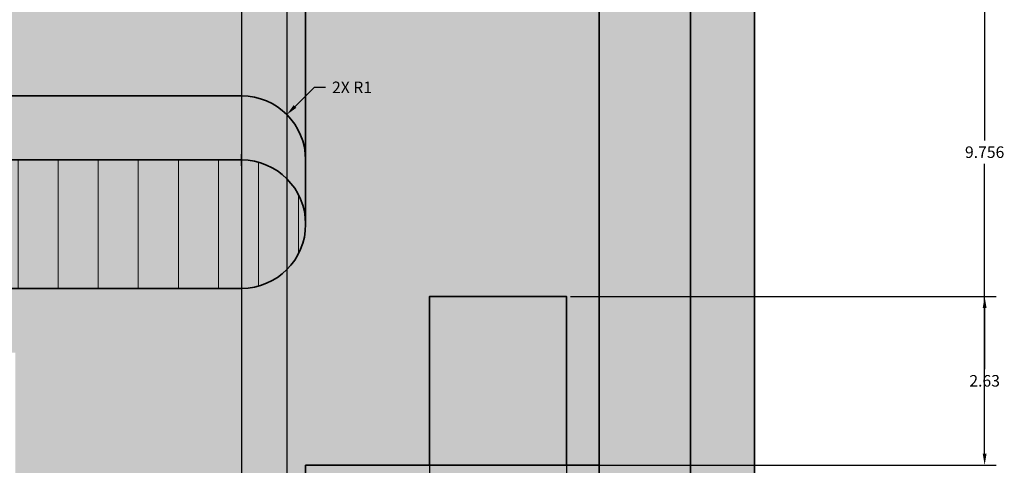
# Model space of a CAD drawing. Units: inches. Extents: x 18 to 59.8, y 2.7 to 81.2.
# Tile 6 of 9: x 44.4 to 59.8, y 38.7 to 45.6. Entities that reach past the tile are written whole.
import ezdxf

# ---------------------------------------------------------------- set-up
doc = ezdxf.new("R2010")
doc.units = ezdxf.units.IN
doc.header["$MEASUREMENT"] = 0
for name, color, linetype, lineweight in [('A-ANNO-DIMS', 2, 'Continuous', 18), ('A-ELEV', 7, 'Continuous', 35), ('A-ELEV-PATT', 8, 'Continuous', 13)]:
    doc.layers.add(name, color=color, linetype=linetype, lineweight=lineweight)
doc.styles.get("Standard").update_dxf_attribs({"font": 'arial.ttf'})
doc.dimstyles.get("Standard").update_dxf_attribs({"dimtxt": 0.18, "dimasz": 0.18, "dimexe": 0.18, "dimexo": 0.0625, "dimgap": 0.09, "dimtad": 0, "dimtih": 1, "dimtoh": 1, "dimdec": 1, "dimzin": 0, "dimdsep": 46, "dimlunit": 3, "dimtxsty": 'Standard', "dimcen": 0.09, "dimadec": 0, "dimazin": 0, "dimtfac": 1, "dimtdec": 1, "dimtofl": 0, "dimtmove": 0, "dimatfit": 3, "dimfxl": 1, "dimtolj": 1, "dimtzin": 0, "dimarcsym": 0})

# ---------------------------------------------------------------- blocks, each defined once
blk = doc.blocks.new('*D17')
at = {"layer": 'A-ANNO-DIMS', "color": 0, "lineweight": -2, "transparency": 16777216}
for p, q in [((53.50256100000002, 48.44074800000003), (59.62997100000005, 48.44074800000003)), ((59.44997100000005, 48.26074800000003), (59.44997100000005, 43.74455863778991)), ((59.44997100000005, 38.86456300000001), (59.44997100000005, 43.38075236221011)), ((53.50256100000002, 38.68456300000001), (59.62997100000006, 38.68456300000001))]:
    blk.add_line(p, q, dxfattribs=at)
at = {"layer": 'A-ANNO-DIMS', "color": 0, "transparency": 16777216}
for points in [[(59.41997100000005, 48.26074800000003), (59.47997100000005, 48.26074800000003), (59.44997100000005, 48.44074800000003)], [(59.41997100000005, 38.86456300000001), (59.47997100000005, 38.86456300000001), (59.44997100000005, 38.68456300000001)]]:
    blk.add_solid(points, dxfattribs=at)
at = {"layer": 'Defpoints', "color": 0, "transparency": 16777216}
for p in [(53.44006100000003, 48.44074800000003), (59.44997100000005, 48.44074800000003), (53.44006100000003, 38.68456300000001)]:
    blk.add_point(p, dxfattribs=at)
at = {"layer": 'A-ANNO-DIMS', "color": 0, "transparency": 16777216, "insert": (59.44997100000005, 43.56265549999998), "char_height": 0.18, "attachment_point": 5}
blk.add_mtext('\\A1;9.756', dxfattribs=at)
blk = doc.blocks.new('*D25')
at = {"layer": 'A-ANNO-DIMS', "color": 0, "lineweight": -2, "transparency": 16777216}
for p, q in [((50.792976, 41.253458), (50.792976, 2.670748000000003)), ((52.926966, 41.253458), (52.926966, 2.670748000000003)), ((50.972976, 2.850747999999999), (51.46510060436562, 2.850747999999999)), ((52.746966, 2.850747999999999), (52.25484139563437, 2.850747999999999))]:
    blk.add_line(p, q, dxfattribs=at)
at = {"layer": 'A-ANNO-DIMS', "color": 0, "transparency": 16777216}
for points in [[(50.972976, 2.880747999999999), (50.972976, 2.820748), (50.792976, 2.850747999999999)], [(52.746966, 2.880747999999999), (52.746966, 2.820748), (52.926966, 2.850747999999999)]]:
    blk.add_solid(points, dxfattribs=at)
at = {"layer": 'Defpoints', "color": 0, "transparency": 16777216}
for p in [(50.792976, 41.315958), (52.926966, 41.315958), (52.926966, 2.850747999999999)]:
    blk.add_point(p, dxfattribs=at)
at = {"layer": 'A-ANNO-DIMS', "color": 0, "transparency": 16777216, "insert": (51.859971, 2.850747999999999), "char_height": 0.18, "attachment_point": 5}
blk.add_mtext('\\A1;2.134', dxfattribs=at)
blk = doc.blocks.new('*D26')
at = {"layer": 'A-ANNO-DIMS', "color": 0, "lineweight": -2, "transparency": 16777216}
for p, q in [((52.98946600000003, 41.31595800000002), (59.62997100000006, 41.31595800000002)), ((59.44997100000005, 41.13595800000001), (59.44997100000005, 40.18222502933153)), ((59.44997100000005, 38.86456300000001), (59.44997100000005, 39.8182959706685)), ((52.98946600000003, 38.68456300000001), (59.62997100000006, 38.68456300000001))]:
    blk.add_line(p, q, dxfattribs=at)
at = {"layer": 'A-ANNO-DIMS', "color": 0, "transparency": 16777216}
for points in [[(59.41997100000005, 41.13595800000001), (59.47997100000005, 41.13595800000001), (59.44997100000005, 41.31595800000002)], [(59.41997100000005, 38.86456300000001), (59.47997100000005, 38.86456300000001), (59.44997100000005, 38.68456300000001)]]:
    blk.add_solid(points, dxfattribs=at)
at = {"layer": 'Defpoints', "color": 0, "transparency": 16777216}
for p in [(52.92696600000002, 41.31595800000002), (59.44997100000005, 41.31595800000002), (52.92696600000002, 38.68456300000001)]:
    blk.add_point(p, dxfattribs=at)
at = {"layer": 'A-ANNO-DIMS', "color": 0, "transparency": 16777216, "insert": (59.44997100000005, 40.00026049999998), "char_height": 0.18, "attachment_point": 5}
blk.add_mtext('\\A1;2.63', dxfattribs=at)
blk = doc.blocks.new('*D51')
at = {"layer": 'A-ANNO-DIMS', "color": 0, "lineweight": -2, "transparency": 16777216}
for p, q in [((34.011642, 44.50324799999999), (34.011642, 81.210748)), ((48.859971, 43.503248), (48.859971, 81.210748)), ((34.191642, 81.03074799999999), (40.98046543587994, 81.03074799999999)), ((48.679971, 81.03074799999999), (41.89114756412005, 81.03074799999999))]:
    blk.add_line(p, q, dxfattribs=at)
at = {"layer": 'A-ANNO-DIMS', "color": 0, "transparency": 16777216}
for points in [[(34.191642, 81.060748), (34.191642, 81.00074799999999), (34.011642, 81.03074799999999)], [(48.679971, 81.060748), (48.679971, 81.00074799999999), (48.859971, 81.03074799999999)]]:
    blk.add_solid(points, dxfattribs=at)
at = {"layer": 'Defpoints', "color": 0, "transparency": 16777216}
for p in [(48.859971, 81.03074799999999), (34.011642, 44.440748), (48.859971, 43.440748)]:
    blk.add_point(p, dxfattribs=at)
at = {"layer": 'A-ANNO-DIMS', "color": 0, "transparency": 16777216, "insert": (41.43580649999999, 81.03074799999999), "char_height": 0.18, "attachment_point": 5}
blk.add_mtext('\\A1;14.848', dxfattribs=at)
blk = doc.blocks.new('*D61')
at = {"layer": 'A-ANNO-DIMS', "color": 0, "lineweight": -2, "transparency": 16777216}
for p, q in [((32.233824, 49.378248), (32.233824, 2.670748000000003)), ((47.859971, 49.378248), (47.859971, 2.670748000000003)), ((32.413824, 2.850747999999999), (39.59180200204638, 2.850747999999999)), ((47.679971, 2.850747999999999), (40.50199299795361, 2.850747999999999))]:
    blk.add_line(p, q, dxfattribs=at)
at = {"layer": 'A-ANNO-DIMS', "color": 0, "transparency": 16777216}
for points in [[(32.413824, 2.880747999999999), (32.413824, 2.820748), (32.233824, 2.850747999999999)], [(47.679971, 2.880747999999999), (47.679971, 2.820748), (47.859971, 2.850747999999999)]]:
    blk.add_solid(points, dxfattribs=at)
at = {"layer": 'Defpoints', "color": 0, "transparency": 16777216}
for p in [(32.233824, 49.440748), (47.859971, 49.440748), (47.859971, 2.850747999999999)]:
    blk.add_point(p, dxfattribs=at)
at = {"layer": 'A-ANNO-DIMS', "color": 0, "transparency": 16777216, "insert": (40.04689749999999, 2.850747999999999), "char_height": 0.18, "attachment_point": 5}
blk.add_mtext('\\A1;15.626', dxfattribs=at)
blk = doc.blocks.new('*D66')
at = {"layer": 'A-ANNO-DIMS', "color": 0, "lineweight": -2, "transparency": 16777216}
for p, q in [((28.803543, 51.378248), (28.803543, 2.670748000000003)), ((48.567078, 51.179103), (48.567078, 2.670748000000003)), ((28.983543, 2.850747999999999), (38.23052195975444, 2.850747999999999)), ((48.387078, 2.850747999999999), (39.14009904024556, 2.850747999999999))]:
    blk.add_line(p, q, dxfattribs=at)
at = {"layer": 'A-ANNO-DIMS', "color": 0, "transparency": 16777216}
for points in [[(28.983543, 2.880747999999999), (28.983543, 2.820748), (28.803543, 2.850747999999999)], [(48.387078, 2.880747999999999), (48.387078, 2.820748), (48.567078, 2.850747999999999)]]:
    blk.add_solid(points, dxfattribs=at)
at = {"layer": 'Defpoints', "color": 0, "transparency": 16777216}
for p in [(28.803543, 51.440748), (48.567078, 51.24160299999999), (48.567078, 2.850747999999999)]:
    blk.add_point(p, dxfattribs=at)
at = {"layer": 'A-ANNO-DIMS', "color": 0, "transparency": 16777216, "insert": (38.6853105, 2.850747999999999), "char_height": 0.18, "attachment_point": 5}
blk.add_mtext('\\A1;19.764', dxfattribs=at)
blk = doc.blocks.new('*D71')
at = {"layer": 'A-ANNO-DIMS', "color": 0, "lineweight": -2, "transparency": 16777216}
for p, q in [((48.99116316341159, 44.57229696346312), (48.6942251490235, 44.27526528903896)), ((49.17116316341159, 44.57229696346312), (48.99116316341159, 44.57229696346312)), ((47.859971, 43.35074800000001), (47.859971, 43.53074800000001)), ((47.769971, 43.44074800000001), (47.94997099999999, 43.44074800000001))]:
    blk.add_line(p, q, dxfattribs=at)
at = {"layer": 'A-ANNO-DIMS', "color": 0, "transparency": 16777216}
blk.add_solid([(48.67300860085034, 44.29647514720953), (48.71544169719665, 44.25405543086838), (48.56696600000001, 44.14796600000001)], dxfattribs=at)
at = {"layer": 'Defpoints', "color": 0, "transparency": 16777216}
for p in [(48.56696600000001, 44.14796600000001), (47.859971, 43.44074800000001)]:
    blk.add_point(p, dxfattribs=at)
at = {"layer": 'A-ANNO-DIMS', "color": 0, "transparency": 16777216, "insert": (49.58383710611282, 44.57229696346312), "char_height": 0.18, "attachment_point": 5}
blk.add_mtext('\\A1;2X R1', dxfattribs=at)

msp = doc.modelspace()

# ---------------------------------------------------------------- hatches: boundary and pattern name
at = {"layer": 'A-ELEV-PATT'}
h = msp.add_hatch(color=256, dxfattribs=at)
h.set_gradient(color1=(255, 255, 255), color2=(199, 200, 202))
h.paths.add_polyline_path([(38.85997087182833, 75.45212783007513, 0.4125526599533602), (36.85997087192615, 77.44074750583997), (21.85997087182832, 77.44074750583995), (21.85997087182832, 22.44074750583995), (22.85997087182833, 22.44074750583995), (48.85997087182833, 22.44074750583996), (48.85997087182833, 30.92342676155402, 0.4074472928332927), (48.33023903111634, 31.44074750583995), (30.40609029701442, 31.44074750583996, -0.7603989452129261), (34.01164157247843, 44.44074750583996), (47.85997087182832, 44.44074750583995, -0.4142135623730951), (48.85997087182833, 43.44074750583994), (48.85997087182833, 48.44074750583995, 0.4142135623730955), (47.85997087182832, 49.44074750583995), (32.23382408177119, 49.44074750583993, -0.2243141867862321), (27.84111392101349, 52.84266085519661, -0.8480128940945467), (38.85997087182833, 61.44074750583993)])
h.paths.add_polyline_path([(55.85997087182832, 77.44074750583995), (54.85997087182832, 77.44074750583997), (54.85997087182832, 22.24074750583996), (55.85997087182832, 22.24074750583995)])
h.paths.add_polyline_path([(54.85997087182832, 51.54074750583995), (53.44006084017791, 51.54074750583996), (53.44006084017792, 29.64074750583996), (54.85997087182832, 29.64074750583996)])
h.paths.add_polyline_path([(54.85997087182832, 61.44074750583993), (53.44006084017791, 57.44074750583993), (53.44006084017791, 51.64074750583996), (54.85997087182832, 51.64074750583996)])
h.paths.add_polyline_path([(54.85997087182832, 29.44074750583995), (54.47100875861361, 29.44074750583995), (54.47100875861361, 22.24074750583996), (54.85997087182832, 22.24074750583996)])
h.paths.add_polyline_path([(55.57447446325177, 22.24074750583995), (54.85997087182832, 22.24074750583996), (54.57447446325178, 22.24074750583996), (53.93466996146642, 21.792542566958), (54.58769880335594, 21.54947740208223)])
h.paths.add_polyline_path([(54.59913950424823, 21.54521903603421), (53.94430429933965, 21.78895655088426), (53.94430429933965, 18.44074750583995), (54.59913950424823, 18.44074750583995)])
h.paths.add_polyline_path([(53.94430429933965, 21.78895655088427), (53.93466996146642, 21.792542566958), (53.58162006229036, 21.54521903603422), (53.58162006229036, 18.44074750583995), (53.94430429933965, 18.44074750583994)])
h.paths.add_polyline_path([(53.36475139777029, 20.69276091189374), (52.89555240690669, 21.06460517556268), (52.89555240690669, 18.44074750583995), (53.3647513977703, 18.44074750583994)])
h.paths.add_polyline_path([(52.89555240690669, 21.06460517556268), (50.57752474318004, 19.44074750583995), (50.57752474318004, 18.44074750583995), (52.89555240690669, 18.44074750583995)])
h.paths.add_polyline_path([(53.58162006229036, 21.54521903603423), (52.89555240690668, 21.06460517556268), (53.3647513977703, 20.69276091189373), (53.58162006229036, 20.84468482967704)])
h.paths.add_polyline_path([(26.81093959479239, 19.44074750583995), (24.96715419074249, 20.84074750583995), (24.96715419074249, 18.44074750583995), (26.81093959479239, 18.44074750583995)])
h.paths.add_polyline_path([(24.96715419074249, 20.84074750583995), (24.41645576890079, 20.84268308307895), (24.41645576890079, 18.44074750583994), (24.96715419074249, 18.44074750583994)])
h.paths.add_polyline_path([(24.41645576890079, 20.84268308307895), (24.41645576890079, 21.25889692219009), (24.05877847081848, 21.5304839605815), (24.03006070560372, 21.51834150822755), (24.03006070560372, 18.44074750583995), (24.41645576890079, 18.44074750583995)])
h.paths.add_polyline_path([(24.03006070560372, 21.51834150822755), (23.41645576890078, 21.2588969221901), (23.41645576890078, 18.44074750583996), (24.03006070560372, 18.44074750583995)])
h.paths.add_polyline_path([(24.03006070560372, 21.51834150822755), (24.05877847081849, 21.53048396058151), (23.12336878669258, 22.24074750583995), (22.12336878669259, 22.24074750583996), (23.41645576890079, 21.2588969221901)])
h.paths.add_polyline_path([(24.41645576890079, 21.2588969221901), (24.41645576890079, 20.84268308307896), (24.96715419074249, 20.84074750583994)])
h.paths.add_polyline_path([(47.85997087182832, 18.44074750583995), (29.85997087182832, 18.44074750583995), (29.85997087182832, 6.440747505839951), (30.85997087182832, 6.440747505839937), (30.85997087182832, 17.44074750583995), (38.85997087182833, 17.44074750583995), (46.85997087182832, 17.44074750583995), (46.85997087182832, 6.440747505839937), (47.85997087182832, 6.440747505839958)])
h.paths.add_polyline_path([(54.57559250001032, 15.2149800477124), (54.57559250001032, 6.440747505839944), (55.85997087182832, 6.440747505839951), (55.85997087182832, 18.44074750583995), (47.85997087182832, 18.44074750583995), (47.85997087182832, 6.440747505839944), (49.14824210254597, 6.440747505839944), (49.14824210254597, 15.2149800477124, -1)])
h = msp.add_hatch(color=256, dxfattribs=at)
h.paths.add_polyline_path([(27.84111392101356, 52.84266085519647, -0.7443789445921651), (36.85997087182832, 61.44074750583993), (38.85997087182833, 61.44074750583993, 0.8480128940945556)])
h.paths.add_polyline_path([(47.85997087182832, 44.44074750583995), (34.01164157247843, 44.44074750583996, 0.7603989452129407), (30.40609029701462, 31.44074750583983, -0.7376245609052545), (34.01164157247731, 43.44074750583994), (47.85997087182831, 43.44074750583994, -0.4142135623730951), (48.85997087182832, 42.44074750583995), (48.85997087182833, 43.44074750583994, 0.4142135623730951)])
h.paths.add_polyline_path([(54.57559250001032, 15.2149800477124), (54.57559250001032, 6.440747505839951), (55.85997087182832, 6.440747505839951), (55.85997087182832, 18.44074750583995), (47.85997087182832, 18.44074750583995), (47.85997087182832, 6.440747505839944), (49.14824210254597, 6.440747505839944), (49.14824210254597, 15.2149800477124, -1)])
h.paths.add_polyline_path([(47.85997087182832, 18.44074750583995), (29.85997087182832, 18.44074750583995), (29.85997087182832, 6.440747505839958), (30.85997087182832, 6.440747505839951), (30.85997087182832, 17.44074750583995), (38.85997087182833, 17.44074750583995), (46.85997087182832, 17.44074750583995), (46.85997087182832, 6.440747505839944), (47.85997087182832, 6.440747505839951)])
h.paths.add_polyline_path([(55.85997087182832, 77.44074750583995), (54.85997087182832, 77.44074750583997), (54.85997087182833, 22.24074750583995), (55.85997087182832, 22.24074750583995)])
h = msp.add_hatch(color=256, dxfattribs=at)
h.dxf.hatch_style = 1
h.paths.add_polyline_path([(54.85997087182832, 69.44074750583995), (38.85997087182833, 69.44074750583995), (38.85997087182833, 61.44074750583995), (54.85997087182832, 61.44074750583994)])
h.paths.add_polyline_path([(54.85997087182833, 61.44074750583994), (38.85997087182833, 61.44074750583995), (36.85997087182832, 61.44074750583993, 0.4434140223301819), (27.69861713021859, 58.44074750583995), (48.85997087182833, 58.44074750583995), (48.85997087182833, 57.44074750583994), (53.44006084017792, 57.44074750583995)])
h.paths.add_polyline_path([(37.49943513222304, 59.93991004599954), (37.49943513222304, 59.81982440572959, -2.410649922227508), (37.11866134610267, 59.81982440572959), (37.11866134610267, 59.93991004599954)], flags=16)
h.paths.add_polyline_path([(42.61253184194623, 59.80122867549901), (42.61253184194623, 59.92131431576897), (42.9933056280666, 59.92131431576897), (42.9933056280666, 59.80122867549901, -2.410649922227521)], flags=16)
h.paths.add_polyline_path([(49.59651616109447, 59.97095150496527), (49.59651616109447, 60.09103714523522), (49.97728994721485, 60.09103714523522), (49.97728994721485, 59.97095150496527, -2.410649922227521)], flags=16)
h.paths.add_polyline_path([(44.46707765301489, 57.04074750583994), (32.6670776530149, 57.04074750583994), (32.6670776530149, 56.04074750583993), (44.46707765301489, 56.04074750583993)])
h.paths.add_polyline_path([(47.85997087182831, 43.44074750583994), (46.85997087182832, 43.44074750583994), (34.0116415724774, 43.44074750583994, 0.2012982920418866), (29.34810857035394, 41.44074750583995), (47.85997087182831, 41.44074750583995, 1)])
h.paths.add_polyline_path([(36.55415719635351, 42.51454569609198), (36.55415719635351, 42.63463133636193), (36.93493098247388, 42.63463133636193), (36.93493098247388, 42.51454569609198, -2.410649922227513)], flags=16)
h.paths.add_polyline_path([(42.93899993637245, 42.54016758592221), (42.93899993637245, 42.66025322619216), (43.31977372249282, 42.66025322619216), (43.31977372249282, 42.54016758592221, -2.410649922227521)], flags=16)
h.paths.add_polyline_path([(54.47100875861361, 29.44074750583995), (48.85997087182833, 29.44074750583995), (48.85997087182833, 22.24074750583995), (54.47100875861361, 22.24074750583995)])
h.paths.add_polyline_path([(54.57447446325178, 22.24074750583996), (23.12336878669258, 22.24074750583996), (26.81093959479238, 19.44074750583996), (50.57752474318006, 19.44074750583996)])
h.paths.add_polyline_path([(54.57559250001032, 15.2149800477124, 1), (49.14824210254597, 15.2149800477124), (49.14824210254597, 6.440747505839958), (54.57559250001032, 6.440747505839965)])
h.paths.add_polyline_path([(49.83226884926398, 12.6020427608384), (49.83226884926398, 9.122455521673542), (49.66565363924473, 9.122455521673537), (49.66565363924473, 12.6020427608384)], flags=16)
h = msp.add_hatch(dxfattribs=at)
h.set_pattern_fill('ANSI31', color=256, scale=5, angle=45, style=0)
h.set_pattern_definition([(90, (0, 0), (-0.6250000000000001, 0), [])])
h.paths.add_polyline_path([(54.85997087182832, 69.44074750583995), (38.85997087182833, 69.44074750583995), (38.85997087182833, 61.44074750583995), (54.85997087182832, 61.44074750583994)])
h.paths.add_polyline_path([(54.85997087182833, 61.44074750583994), (38.85997087182833, 61.44074750583995), (36.85997087182832, 61.44074750583993, 0.4434140223301819), (27.69861713021859, 58.44074750583995), (48.85997087182833, 58.44074750583995), (48.85997087182833, 57.44074750583994), (53.44006084017792, 57.44074750583995)])
h.paths.add_polyline_path([(37.16613704638868, 59.85769359025997), (37.11866134610267, 59.85769359025997), (37.11866134610267, 59.93991004599954), (37.49943513222304, 59.93991004599954), (37.49943513222304, 59.85769359025997), (37.45195943193702, 59.85769359025997, -3.476462016968403)], flags=16)
h.paths.add_polyline_path([(42.66000754223224, 59.8390978600294), (42.61253184194623, 59.8390978600294), (42.61253184194623, 59.92131431576897), (42.9933056280666, 59.92131431576897), (42.9933056280666, 59.8390978600294), (42.94582992778058, 59.8390978600294, -3.47646201696846)], flags=16)
h.paths.add_polyline_path([(49.64399186138049, 60.00882068949565), (49.59651616109447, 60.00882068949565), (49.59651616109447, 60.09103714523522), (49.97728994721485, 60.09103714523522), (49.97728994721485, 60.00882068949565), (49.92981424692883, 60.00882068949565, -3.476462016968434)], flags=16)
h.paths.add_polyline_path([(44.46707765301489, 57.04074750583994), (32.6670776530149, 57.04074750583994), (32.6670776530149, 56.04074750583993), (44.46707765301489, 56.04074750583993)])
h.paths.add_polyline_path([(47.85997087182831, 43.44074750583994), (46.85997087182832, 43.44074750583994), (34.0116415724774, 43.44074750583994, 0.2012982920418866), (29.34810857035394, 41.44074750583995), (47.85997087182831, 41.44074750583995, 1)])
h.paths.add_polyline_path([(36.60163289663952, 42.55241488062237), (36.55415719635351, 42.55241488062236), (36.55415719635351, 42.63463133636193), (36.93493098247388, 42.63463133636193), (36.93493098247388, 42.55241488062236), (36.88745528218787, 42.55241488062236, -3.476462016968307)], flags=16)
h.paths.add_polyline_path([(42.98647563665846, 42.5780367704526), (42.93899993637245, 42.5780367704526), (42.93899993637245, 42.66025322619216), (43.31977372249282, 42.66025322619216), (43.31977372249282, 42.57803677045259), (43.2722980222068, 42.57803677045259, -3.476462016968351)], flags=16)
h.paths.add_polyline_path([(54.47100875861361, 29.44074750583995), (48.85997087182833, 29.44074750583995), (48.85997087182833, 22.24074750583995), (54.47100875861361, 22.24074750583994)])
h.paths.add_polyline_path([(54.57447446325179, 22.24074750583995), (23.12336878669258, 22.24074750583995), (26.81093959479238, 19.44074750583996), (50.57752474318005, 19.44074750583996)])
h.paths.add_polyline_path([(54.57559250001032, 15.2149800477124, 1), (49.14824210254597, 15.2149800477124), (49.14824210254597, 6.440747505839958), (54.57559250001032, 6.440747505839944)])
h.paths.add_polyline_path([(49.83226884926398, 9.122455521673542), (49.66565363924473, 9.122455521673537), (49.66565363924473, 12.60204276083839), (49.83226884926398, 12.6020427608384)], flags=16)
at = {"layer": 'A-ELEV-PATT', "transparency": 33554620}
h = msp.add_hatch(color=256, dxfattribs=at)
h.set_gradient(color1=(147, 149, 152))
edge = h.paths.add_edge_path()
edge.add_line((32.5670776530149, 55.94074750583994), (32.5670776530149, 57.14074750583994))
edge.add_line((32.5670776530149, 57.14074750583994), (44.5670776530149, 57.14074750583994))
edge.add_line((44.5670776530149, 57.14074750583994), (44.5670776530149, 55.94074750583994))
edge.add_line((44.5670776530149, 55.94074750583994), (44.56707765301487, 51.54074750583998))
edge.add_line((44.56707765301487, 51.54074750583998), (47.92075940082271, 51.54074750583998))
edge.add_spline(control_points=[(47.92075940082271, 51.54074750583998), (48.15238228194087, 51.51452682454292), (48.35972996747788, 51.37806491819363), (48.56707765301488, 51.24160301184435)], knot_values=[0, 0, 0, 0, 0.7121900809507601, 0.7121900809507601, 0.7121900809507601, 0.7121900809507601], degree=3, periodic=0)
edge.add_line((48.56707765301488, 51.24160301184435), (48.56707765301488, 49.14785428702649))
edge.add_arc((47.85997087182832, 48.44074750583995), 1, 5.739170477267294, 44.999999999999375, ccw=False)
edge.add_line((48.85495830893494, 48.54074750583996), (48.85997087182833, 48.54074750583996))
edge.add_line((48.85997087182833, 48.54074750583996), (48.85997087182833, 49.44074750583995))
edge.add_line((48.85997087182833, 49.44074750583995), (48.85997087182833, 58.44074750583995))
edge.add_line((48.85997087182833, 58.44074750583995), (27.6986171302186, 58.44074750583995))
edge.add_arc((33.63815495998532, 55.79107886226907), 6.503756879831279, 155.9580213816849, 220.80747886606)
edge.add_line((28.71539791616241, 51.54074750583994), (32.5670776530149, 51.54074750583994))
edge.add_line((32.5670776530149, 51.54074750583994), (32.5670776530149, 55.94074750583994))
edge = h.paths.add_edge_path()
edge.add_line((32.33023903111487, 40.44074750583996), (35.33023903111486, 40.44074750583996))
edge.add_line((35.33023903111486, 40.44074750583996), (38.33023903111485, 40.44074750583996))
edge.add_line((38.33023903111485, 40.44074750583996), (41.33023903111483, 40.44074750583996))
edge.add_line((41.33023903111483, 40.44074750583996), (44.33023903111482, 40.44074750583996))
edge.add_line((44.33023903111482, 40.44074750583996), (44.33023903111482, 33.83364072465343))
edge.add_line((44.33023903111482, 33.83364072465343), (47.68392077892264, 33.83364072465344))
edge.add_spline(control_points=[(47.68392077892267, 33.83364072465344), (47.91554366004082, 33.80742004335637), (48.12289134557783, 33.67095813700708), (48.33023903111483, 33.5344962306578)], knot_values=[0, 0, 0, 0, 0.7121900809507601, 0.7121900809507601, 0.7121900809507601, 0.7121900809507601], degree=3, periodic=0)
edge.add_line((48.33023903111483, 33.5344962306578), (48.33023903111483, 31.44074750583995))
edge.add_arc((48.3303844405005, 30.91101568508362), 0.5297318407134953, 1.3425044870115812, 90.01572747485528, ccw=False)
edge.add_line((48.85997087182833, 30.92342676155392), (48.85997087182833, 38.68456317332766))
edge.add_line((48.85997087182833, 38.68456317332766), (50.79297551695841, 38.68456317332766))
edge.add_line((50.79297551695841, 38.68456317332766), (50.79297551695841, 41.31595823441438))
edge.add_line((50.79297551695841, 41.31595823441438), (52.92696622669824, 41.31595823441438))
edge.add_line((52.92696622669824, 41.31595823441438), (52.92696622669824, 38.68456317332766))
edge.add_line((52.92696622669824, 38.68456317332766), (53.44006084017791, 38.68456317332766))
edge.add_line((53.44006084017791, 38.68456317332766), (53.44006084017791, 48.44074750583995))
edge.add_line((53.44006084017791, 48.44074750583995), (48.85997087182833, 48.44074750583995))
edge.add_line((48.85997087182833, 48.44074750583995), (48.85997087182832, 42.44074750583995))
edge.add_arc((47.85997087182831, 42.44074750583995), 1, -90, 0, ccw=False)
edge.add_line((47.85997087182831, 41.44074750583995), (29.34810857035394, 41.44074750583995))
edge.add_arc((34.06310194306089, 36.8836189221075), 6.557330511217327, 135.9754091201121, 207.7183105881144)
edge.add_line((28.25825772220566, 33.83364072465339), (32.33023903111487, 33.83364072465341))
edge.add_line((32.33023903111487, 33.83364072465341), (32.33023903111487, 40.44074750583996))
h.paths.add_polyline_path([(53.44006084017791, 57.44074750583995), (48.85997087182833, 57.44074750583994), (48.85997087182833, 51.64074750583996), (53.44006084017791, 51.64074750583996)])
h.paths.add_polyline_path([(29.56707765301488, 51.44074750583992), (28.80354322363853, 51.44074750583992, 0.040450980236505), (29.56707765301488, 50.71907894974708)], flags=17)
h.paths.add_polyline_path([(30.06707765301488, 51.44074750583992), (29.56707765301488, 51.44074750583992), (29.56707765301488, 50.71907894974708, 0.0237787432624053), (30.06707765301488, 50.35543166808938)], flags=17)
h.paths.add_polyline_path([(30.56707765301487, 51.44074750583993), (30.06707765301488, 51.44074750583992), (30.06707765301488, 50.35543166808938, 0.0223728768734236), (30.56707765301488, 50.05807461261393)], flags=17)
h.paths.add_polyline_path([(31.06707765301487, 51.44074750583993), (30.56707765301487, 51.44074750583993), (30.56707765301488, 50.05807461261393, 0.021345047641792), (31.06707765301488, 49.8171007041625)], flags=17)
h.paths.add_polyline_path([(31.56707765301487, 51.44074750583993), (31.06707765301487, 51.44074750583993), (31.06707765301488, 49.8171007041625, 0.0205857748313696), (31.56707765301488, 49.62589497689267)], flags=17)
h.paths.add_polyline_path([(32.06707765301488, 51.44074750583993), (31.56707765301487, 51.44074750583993), (31.56707765301488, 49.62589497689267, 0.0200299041308402), (32.06707765301488, 49.47993240164282)], flags=17)
h.paths.add_polyline_path([(32.5670776530149, 51.44074750583993), (32.06707765301488, 51.44074750583993), (32.06707765301488, 49.47993240164282, 0.0065845078177353), (32.23382408177119, 49.44074750583993), (32.5670776530149, 49.44074750583993)], flags=17)
h.paths.add_polyline_path([(45.06707765301486, 51.44074750583996), (44.56707765301487, 51.44074750583996), (44.56707765301487, 49.44074750583995), (45.06707765301488, 49.44074750583995)], flags=17)
h.paths.add_polyline_path([(45.56707765301488, 51.44074750583996), (45.06707765301486, 51.44074750583996), (45.06707765301488, 49.44074750583995), (45.56707765301488, 49.44074750583995)], flags=17)
h.paths.add_polyline_path([(46.06707765301488, 51.44074750583996), (45.56707765301488, 51.44074750583996), (45.56707765301488, 49.44074750583995), (46.06707765301488, 49.44074750583995)], flags=17)
h.paths.add_polyline_path([(46.56707765301487, 51.44074750583996), (46.06707765301488, 51.44074750583996), (46.06707765301488, 49.44074750583995), (46.56707765301487, 49.44074750583995)], flags=17)
h.paths.add_polyline_path([(47.06707765301487, 51.44074750583996), (46.56707765301487, 51.44074750583996), (46.56707765301487, 49.44074750583995), (47.06707765301487, 49.44074750583995)], flags=17)
h.paths.add_polyline_path([(47.56707765301487, 51.44074750583996), (47.06707765301487, 51.44074750583996), (47.06707765301487, 49.44074750583995), (47.56707765301488, 49.44074750583995)], flags=17)
edge = h.paths.add_edge_path(flags=17)
edge.add_spline(control_points=[(48.06707765301273, 51.41840713962396), (48.02172392661717, 51.43105064440995), (47.97524027779975, 51.4389035969284), (47.92733930740307, 51.44074750583996)], knot_values=[0.5701039528936005, 0.5701039528936005, 0.5701039528936005, 0.5701039528936005, 0.7151116034373463, 0.7151116034373463, 0.7151116034373463, 0.7151116034373644], degree=3, periodic=0)
edge.add_line((47.92733930740307, 51.44074750583996), (47.56707765301487, 51.44074750583996))
edge.add_line((47.56707765301487, 51.44074750583996), (47.56707765301488, 49.44074750583995))
edge.add_line((47.56707765301488, 49.44074750583995), (47.85997087182832, 49.44074750583995))
edge.add_arc((47.85997087182832, 48.44074750583995), 1, 78.04714410929728, 90, ccw=False)
edge.add_line((48.06707765301489, 49.41906584931846), (48.06707765301488, 51.41840713962341))
edge = h.paths.add_edge_path(flags=17)
edge.add_spline(control_points=[(48.56707765301488, 51.12118615879595), (48.40623273758901, 51.24494240176197), (48.24538782216315, 51.36869864472799), (48.06707765301273, 51.41840713962396)], knot_values=[0, 0, 0, 0, 0.5701039528936005, 0.5701039528936005, 0.5701039528936005, 0.5701039528936005], degree=3, periodic=0)
edge.add_line((48.06707765301488, 51.41840713962327), (48.06707765301489, 49.41906584931846))
edge.add_arc((47.85997087182832, 48.44074750583995), 1, 44.999999999999375, 78.04714410929728, ccw=False)
edge.add_line((48.56707765301488, 49.14785428702649), (48.56707765301488, 51.12118615879595))
h.paths.add_polyline_path([(49.35997087182833, 51.54074750583996), (48.85997087182833, 51.54074750583996), (48.85997087182833, 49.44074750583995), (48.85997087182833, 48.54074750583996), (49.35997087182833, 48.54074750583996)])
h.paths.add_polyline_path([(49.85997087182834, 51.54074750583996), (49.35997087182833, 51.54074750583996), (49.35997087182833, 48.54074750583996), (49.85997087182833, 48.54074750583996)])
h.paths.add_polyline_path([(50.35997087182834, 51.54074750583996), (49.85997087182834, 51.54074750583996), (49.85997087182833, 48.54074750583996), (50.35997087182833, 48.54074750583996)])
h.paths.add_polyline_path([(50.85997087182834, 51.54074750583996), (50.35997087182834, 51.54074750583996), (50.35997087182832, 48.54074750583996), (50.85997087182833, 48.54074750583996)])
h.paths.add_polyline_path([(51.35997087182833, 51.54074750583996), (50.85997087182834, 51.54074750583996), (50.85997087182833, 48.54074750583996), (51.35997087182833, 48.54074750583996)])
h.paths.add_polyline_path([(51.85997087182833, 51.54074750583996), (51.35997087182833, 51.54074750583996), (51.35997087182833, 48.54074750583995), (51.85997087182832, 48.54074750583995)])
h.paths.add_polyline_path([(52.35997087182834, 51.54074750583995), (51.85997087182833, 51.54074750583996), (51.85997087182832, 48.54074750583995), (52.35997087182834, 48.54074750583995)])
h.paths.add_polyline_path([(52.85997087182835, 51.54074750583995), (52.35997087182834, 51.54074750583995), (52.35997087182834, 48.54074750583995), (52.85997087182833, 48.54074750583995)])
h.paths.add_polyline_path([(53.35997087182834, 51.54074750583995), (52.85997087182835, 51.54074750583995), (52.85997087182833, 48.54074750583995), (53.35997087182834, 48.54074750583995)])
h.paths.add_polyline_path([(53.44006084017792, 38.68456317332766), (48.85997087182833, 38.68456317332766), (48.85997087182833, 30.92342676155392), (48.85997087182833, 29.64074750583995), (53.44006084017792, 29.64074750583994)])
h.paths.add_polyline_path([(28.83023903111483, 33.73364072465339), (28.31190895474052, 33.73364072465339, 0.0364451520675395), (28.83023903111484, 32.93194469741221)], flags=17)
h.paths.add_polyline_path([(29.33023903111483, 33.73364072465339), (28.83023903111483, 33.73364072465339), (28.83023903111484, 32.9319446974122, 0.0294200839082379), (29.33023903111484, 32.34505173740402)], flags=17)
h.paths.add_polyline_path([(29.83023903111483, 33.73364072465339), (29.33023903111483, 33.73364072465339), (29.33023903111484, 32.34505173740402, 0.0261691093073466), (29.83023903111483, 31.87548004603654)], flags=17)
h.paths.add_polyline_path([(30.33023903111483, 33.73364072465339), (29.83023903111483, 33.73364072465339), (29.83023903111483, 31.87548004603654, 0.0240262665661449), (30.33023903111483, 31.49248565404972)], flags=17)
h.paths.add_polyline_path([(30.83023903111483, 33.73364072465339), (30.33023903111483, 33.73364072465339), (30.33023903111483, 31.49248565404973, 0.0035005678246481), (30.40609029701443, 31.44074750583996), (30.83023903111484, 31.44074750583996)], flags=17)
h.paths.add_polyline_path([(31.33023903111483, 33.73364072465339), (30.83023903111483, 33.73364072465339), (30.83023903111484, 31.44074750583996), (31.33023903111483, 31.44074750583996)], flags=17)
h.paths.add_polyline_path([(31.83023903111483, 33.73364072465339), (31.33023903111483, 33.73364072465339), (31.33023903111483, 31.44074750583996), (31.83023903111483, 31.44074750583996)], flags=17)
h.paths.add_polyline_path([(32.33023903111487, 33.7336407246534), (31.83023903111483, 33.7336407246534), (31.83023903111483, 31.44074750583996), (32.33023903111487, 31.44074750583996)], flags=17)
h.paths.add_polyline_path([(44.83023903111482, 33.73364072465341), (44.33023903111482, 33.73364072465341), (44.33023903111482, 31.44074750583995), (44.83023903111483, 31.44074750583995)], flags=17)
h.paths.add_polyline_path([(45.33023903111483, 33.73364072465341), (44.83023903111482, 33.73364072465341), (44.83023903111483, 31.44074750583996), (45.33023903111483, 31.44074750583995)], flags=17)
h.paths.add_polyline_path([(45.83023903111483, 33.73364072465341), (45.33023903111483, 33.73364072465341), (45.33023903111483, 31.44074750583996), (45.83023903111483, 31.44074750583995)], flags=17)
h.paths.add_polyline_path([(46.33023903111483, 33.73364072465342), (45.83023903111483, 33.73364072465342), (45.83023903111483, 31.44074750583995), (46.33023903111482, 31.44074750583996)], flags=17)
h.paths.add_polyline_path([(46.83023903111482, 33.73364072465342), (46.33023903111483, 33.73364072465342), (46.33023903111482, 31.44074750583996), (46.83023903111482, 31.44074750583995)], flags=17)
h.paths.add_polyline_path([(47.33023903111482, 33.73364072465342), (46.83023903111482, 33.73364072465341), (46.83023903111482, 31.44074750583996), (47.33023903111484, 31.44074750583996)], flags=17)
edge = h.paths.add_edge_path(flags=16)
edge.add_spline(control_points=[(47.83023903111267, 33.71130035843739), (47.78488530471712, 33.7239438632234), (47.7384016558997, 33.73179681574185), (47.690500685503, 33.73364072465343)], knot_values=[0.5701039528936152, 0.5701039528936152, 0.5701039528936152, 0.5701039528936152, 0.7151116034373552, 0.7151116034373552, 0.7151116034373552, 0.7151116034373644], degree=3, periodic=0)
edge.add_line((47.69050068550314, 33.73364072465342), (47.33023903111482, 33.73364072465342))
edge.add_line((47.33023903111482, 33.73364072465342), (47.33023903111484, 31.44074750583995))
edge.add_line((47.33023903111484, 31.44074750583995), (47.83023903111484, 31.44074750583995))
edge.add_line((47.83023903111484, 31.44074750583995), (47.83023903111483, 33.71130035843684))
h.paths.add_polyline_path([(48.85997087182833, 38.68456317332766), (50.79297551695841, 38.68456317332766), (50.79297551695841, 41.31595823441438), (52.92696622669824, 41.31595823441438), (52.92696622669824, 38.68456317332766), (53.44006084017791, 38.68456317332766), (53.44006084017791, 48.44074750583995), (48.85997087182833, 48.44074750583995), (48.85997087182832, 42.44074750583995, -0.414213562373094), (47.85997087182831, 41.44074750583995), (29.34810857035394, 41.44074750583995, 0.3236799116418651), (28.25825772220566, 33.83364072465339), (32.33023903111487, 33.83364072465341), (32.33023903111487, 40.44074750583996), (35.33023903111486, 40.44074750583996), (38.33023903111485, 40.44074750583996), (41.33023903111483, 40.44074750583996), (44.33023903111482, 40.44074750583996), (44.33023903111482, 33.83364072465343), (28.25825772220566, 33.83364072465339, 0.0043266617348909), (28.31190895474052, 33.73364072465339), (28.83023903111483, 33.73364072465339), (29.33023903111483, 33.73364072465339), (29.83023903111483, 33.73364072465339), (30.33023903111483, 33.73364072465339), (30.83023903111483, 33.73364072465339), (31.33023903111483, 33.73364072465339), (31.83023903111483, 33.73364072465339), (32.33023903111487, 33.7336407246534), (47.33023903111482, 33.73364072465342), (47.33023903111484, 31.44074750583995), (47.83023903111484, 31.44074750583995), (48.33023903111591, 31.44074750583995, -0.4074472928335827), (48.85997087182833, 30.92342676155392)])
edge = h.paths.add_edge_path(flags=0)
edge.add_spline(control_points=[(47.83023903111267, 33.71130035843739), (47.78488530471713, 33.7239438632234), (47.73840165589972, 33.73179681574185), (47.69050068550303, 33.73364072465341)], knot_values=[0.5701039528936152, 0.5701039528936152, 0.5701039528936152, 0.5701039528936152, 0.7151116034373257, 0.7151116034373257, 0.7151116034373257, 0.7151116034373644], degree=3, periodic=0)
edge.add_line((47.69050068550293, 33.73364072465342), (47.33023903111482, 33.73364072465342))
edge.add_line((47.33023903111482, 33.73364072465342), (47.33023903111484, 31.44074750583995))
edge.add_line((47.33023903111484, 31.44074750583995), (47.83023903111484, 31.44074750583995))
edge.add_line((47.83023903111484, 31.44074750583995), (47.83023903111483, 33.71130035843687))
h = msp.add_hatch(color=256, dxfattribs=at)
h.set_gradient(color1=(147, 149, 152))
edge = h.paths.add_edge_path()
edge.add_line((44.33023903111482, 33.83364072465343), (47.68392077892268, 33.83364072465344))
edge.add_spline(control_points=[(47.68392077892267, 33.83364072465344), (47.91554366004082, 33.80742004335637), (48.12289134557783, 33.67095813700708), (48.33023903111483, 33.5344962306578)], knot_values=[0, 0, 0, 0, 0.7121900809507601, 0.7121900809507601, 0.7121900809507601, 0.7121900809507601], degree=3, periodic=0)
edge.add_line((48.33023903111483, 33.5344962306578), (48.33023903111483, 31.44074750583995))
edge.add_arc((48.3303844405005, 30.91101568508362), 0.5297318407134953, 1.3425044870177203, 90.01572747485528, ccw=False)
edge.add_line((48.85997087182833, 30.92342676155398), (48.85997087182833, 38.68456317332766))
edge.add_line((48.85997087182833, 38.68456317332766), (50.79297551695841, 38.68456317332766))
edge.add_line((50.79297551695841, 38.68456317332766), (50.79297551695841, 41.31595823441438))
edge.add_line((50.79297551695841, 41.31595823441438), (52.92696622669824, 41.31595823441438))
edge.add_line((52.92696622669824, 41.31595823441438), (52.92696622669824, 38.68456317332766))
edge.add_line((52.92696622669824, 38.68456317332766), (53.44006084017791, 38.68456317332766))
edge.add_line((53.44006084017791, 38.68456317332766), (53.44006084017791, 48.44074750583995))
edge.add_line((53.44006084017791, 48.44074750583995), (48.85997087182833, 48.44074750583995))
edge.add_line((48.85997087182833, 48.44074750583995), (48.85997087182832, 42.44074750583995))
edge.add_arc((47.85997087182831, 42.44074750583995), 1, -90, 0, ccw=False)
edge.add_line((47.85997087182831, 41.44074750583995), (29.34810857035394, 41.44074750583995))
edge.add_arc((34.06310194306089, 36.8836189221075), 6.557330511217328, 135.9754091201121, 207.7183105881144)
edge.add_line((28.25825772220566, 33.83364072465339), (32.33023903111487, 33.8336407246534))
edge.add_line((32.33023903111487, 33.8336407246534), (32.33023903111487, 40.44074750583996))
edge.add_line((32.33023903111487, 40.44074750583996), (35.33023903111486, 40.44074750583996))
edge.add_line((35.33023903111486, 40.44074750583996), (38.33023903111485, 40.44074750583996))
edge.add_line((38.33023903111485, 40.44074750583996), (41.33023903111483, 40.44074750583996))
edge.add_line((41.33023903111483, 40.44074750583996), (44.33023903111482, 40.44074750583996))
edge.add_line((44.33023903111482, 40.44074750583996), (44.33023903111482, 33.83364072465343))
at = {"layer": 'A-ELEV-PATT'}
msp.add_hatch(color=256, dxfattribs=at).paths.add_polyline_path([(52.92696622669824, 41.31595823441438), (50.79297551695841, 41.31595823441438), (50.79297551695841, 38.68456317332766), (52.92696622669824, 38.68456317332766)])

# ---------------------------------------------------------------- linework, layer by layer
at = {"layer": 'A-ELEV'}
for p, q in [((54.85997087182833, 22.24074750583995), (54.85997087182832, 77.44074750583995)), ((55.85997087182832, 77.44074750583994), (55.85997087182832, 22.24074750583995)), ((48.85997087182833, 42.44074750583995), (48.85997087182833, 58.44074750583994)), ((53.44006084017791, 57.44074750583996), (53.44006084017792, 29.64074750583995)), ((47.85997087182832, 44.44074750583995), (34.01164157247843, 44.44074750583995)), ((47.85997087182831, 43.44074750583994), (34.01164157247755, 43.44074750583994)), ((47.85997087182832, 43.44074750583994), (46.85997087182832, 43.44074750583994)), ((47.85997087182831, 41.44074750583995), (29.34810857035394, 41.44074750583995)), ((48.85997087182833, 22.24074750583996), (48.85997087182833, 38.68456317332766))]:
    msp.add_line(p, q, dxfattribs=at)
msp.add_lwpolyline([(50.79297551695841, 38.68456317332766), (52.92696622669824, 38.68456317332766), (52.92696622669824, 41.31595823441438), (50.79297551695841, 41.31595823441438)], close=True, dxfattribs=at)
msp.add_lwpolyline([(53.44006084017792, 38.68456317332766), (48.85997087182833, 38.68456317332766), (48.85997087182833, 29.64074750583995), (54.85997087182832, 29.64074750583995), (54.85997087182832, 38.68456317332766)], dxfattribs=at)
for centre, radius, start in [((47.85997087182832, 43.44074750583994), 1, 0), ((47.85997087182831, 42.44074750583995), 1.000000000000003, 270)]:
    msp.add_arc(centre, radius, start, 90, dxfattribs=at)

# ---------------------------------------------------------------- dimensions: what is measured, and where the dimension line sits
at = {"layer": 'A-ANNO-DIMS'}
for base, p1, p2, picture, middle in [((48.859971, 81.03074799999999), (34.011642, 44.440748), (48.859971, 43.440748), '*D51', (41.43580649999999, 81.03074799999999)), ((48.567078, 2.850747999999999), (28.803543, 51.440748), (48.567078, 51.24160299999999), '*D66', (38.6853105, 2.850747999999999)), ((47.859971, 2.850747999999999), (32.233824, 49.440748), (47.859971, 49.440748), '*D61', (40.04689749999999, 2.850747999999999)), ((52.926966, 2.850747999999999), (50.792976, 41.315958), (52.926966, 41.315958), '*D25', (51.859971, 2.850747999999999))]:
    dim = msp.add_linear_dim(base=base, p1=p1, p2=p2, dimstyle='Standard', override={"dimdec": 3, "dimlfac": 1, "dimrnd": 0, "dimzin": 0, "dimdsep": 46, "dimlunit": 2}, dxfattribs=at)
    dim.commit()
    dim.dimension.update_dxf_attribs({"geometry": picture, "text_midpoint": middle})
for base, p1, p2, override, picture, middle in [((59.44997100000005, 48.44074800000003), (53.440061, 38.684563), (53.440061, 48.440748), {"dimdec": 3, "dimlfac": 1, "dimrnd": 0, "dimzin": 0, "dimdsep": 46, "dimlunit": 2}, '*D17', (59.44997100000005, 43.56265549999998)), ((59.44997100000005, 41.31595800000002), (52.926966, 38.684563), (52.926966, 41.315958), {"dimdec": 2, "dimlfac": 1, "dimrnd": 0, "dimzin": 0, "dimdsep": 46, "dimlunit": 2}, '*D26', (59.44997100000005, 40.00026049999998))]:
    dim = msp.add_linear_dim(base=base, p1=p1, p2=p2, angle=90, dimstyle='Standard', override=override, dxfattribs=at)
    dim.commit()
    dim.dimension.update_dxf_attribs({"geometry": picture, "text_midpoint": middle})
dim = msp.add_radius_dim(center=(47.859971, 43.44074800000001), mpoint=(48.56696600000001, 44.14796600000001), text='2X <>', dimstyle='Standard', override={"dimdec": 0, "dimlfac": 1, "dimrnd": 0, "dimzin": 0, "dimdsep": 46, "dimlunit": 2}, dxfattribs=at)
dim.commit()
dim.dimension.update_dxf_attribs({"geometry": '*D71', "text_midpoint": (49.58383710611282, 44.57229696346312), "dimtype": 164})

doc.saveas('drawing.dxf')
